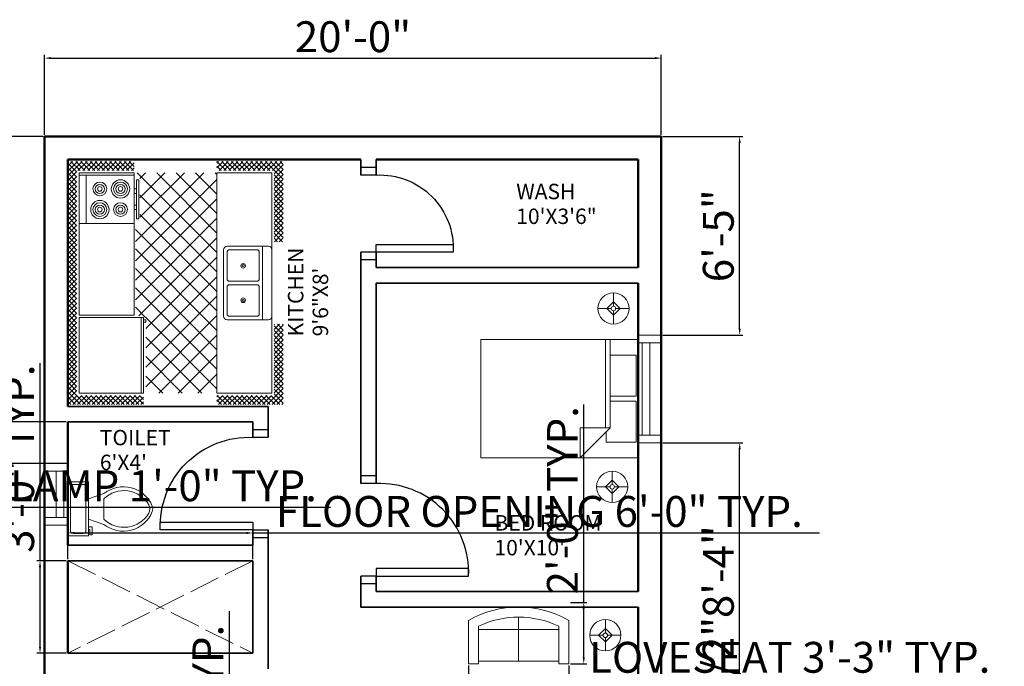
# Model space of a CAD drawing. Units: inches. Extents: x 2296 to 3335, y 495 to 1294.
# Tile 7 of 7: x 2952 to 3335, y 862 to 1113. Entities that reach past the tile are written whole.
import ezdxf

# ---------------------------------------------------------------- set-up
doc = ezdxf.new("R2010")
doc.units = ezdxf.units.IN
doc.linetypes.add('ACAD_ISO02W100', pattern=[15, 12, -3])
for name, color, linetype, lineweight in [('A-ANNO-DIMS', 2, 'Continuous', 18), ('A-AREA-IDEN', 7, 'Continuous', 18), ('A-FLOR-FIXT', 8, 'Continuous', 18), ('A-FLOR-OPEN', 7, 'ACAD_ISO02W100', 18), ('DOORS', 1, 'Continuous', 25), ('E-LITE', 2, 'Continuous', 18), ('FURNITURE', 2, 'Continuous', 18), ('INNER WALL', 6, 'Continuous', 35), ('OUTER WALL', 5, 'Continuous', 50), ('P-FIXT', 4, 'Continuous', 18), ('VENTILATOR', 4, 'Continuous', 18), ('WINDOWS', 3, 'Continuous', 18)]:
    doc.layers.add(name, color=color, linetype=linetype, lineweight=lineweight)
doc.styles.get("Standard").update_dxf_attribs({"font": 'arial.ttf'})
doc.dimstyles.new('ISO-25', dxfattribs={"dimtxt": 12, "dimasz": 2.5, "dimexe": 1.25, "dimexo": 0.625, "dimtad": 1, "dimdec": 1, "dimlunit": 3, "dimtxsty": 'Standard', "dimcen": 2.5, "dimadec": 0, "dimazin": 0, "dimtfac": 1, "dimtdec": 1, "dimtmove": 0, "dimatfit": 3, "dimfxl": 1, "dimarcsym": 0})

# ---------------------------------------------------------------- blocks, each defined once
blk = doc.blocks.new('Kitchen Layout - 7 x 8 ft')
for p, q in [((-5, 81.32), (2.68, 89)), ((-5, 83.44), (0.56, 89)), ((-5, 85.56), (-1.56, 89)), ((-5, 87.68), (-3.68, 89)), ((-1, 84.97), (-5, 88.97)), ((-1, 82.85), (-5, 86.85)), ((1.09, 85), (-2.91, 89)), ((3.21, 85), (-0.79, 89)), ((0.81, 85), (4.81, 89)), ((5.34, 85), (1.34, 89)), ((2.93, 85), (6.93, 89)), ((7.46, 85), (3.46, 89)), ((5.05, 85), (9.05, 89)), ((9.58, 85), (5.58, 89)), ((7.17, 85), (11.17, 89)), ((11.7, 85), (7.7, 89)), ((9.29, 85), (13.29, 89)), ((13.82, 85), (9.82, 89)), ((11.41, 85), (15.41, 89)), ((15.94, 85), (11.94, 89)), ((13.53, 85), (17.53, 89)), ((18.06, 85), (14.06, 89)), ((15.65, 85), (19.65, 89)), ((20.18, 85), (16.18, 89)), ((17.78, 85), (21.78, 89)), ((22.31, 85), (18.31, 89)), ((19.9, 85), (23.9, 89)), ((24.43, 85), (20.43, 89)), ((22.02, 85), (26.02, 89)), ((26.55, 85), (22.55, 89)), ((24.14, 85), (28.14, 89)), ((28.67, 85), (24.67, 89)), ((26.26, 85), (30.26, 89)), ((30.79, 85), (26.79, 89)), ((28.38, 85), (32.38, 89)), ((32.91, 85), (28.91, 89)), ((30.5, 85), (34.5, 89)), ((35.03, 85), (31.03, 89)), ((32.63, 85), (36.63, 89)), ((37.16, 85), (33.16, 89)), ((34.75, 85), (38.75, 89)), ((39.28, 85), (35.28, 89)), ((36.87, 85), (40.87, 89)), ((41.4, 85), (37.4, 89)), ((38.99, 85), (42.99, 89)), ((43.52, 85), (39.52, 89)), ((41.11, 85), (45.11, 89)), ((45.64, 85), (41.64, 89)), ((43.23, 85), (47.23, 89)), ((47.76, 85), (43.76, 89)), ((45.35, 85), (49.35, 89)), ((49.88, 85), (45.88, 89)), ((47.47, 85), (51.47, 89)), ((52, 85), (48, 89)), ((49.6, 85), (53.6, 89)), ((54.13, 85), (50.13, 89)), ((51.72, 85), (55.72, 89)), ((56.25, 85), (52.25, 89)), ((53.84, 85), (57.84, 89)), ((58.37, 85), (54.37, 89)), ((55.96, 85), (59.96, 89)), ((60.49, 85), (56.49, 89)), ((58.08, 85), (62.08, 89)), ((62.61, 85), (58.61, 89)), ((60.2, 85), (64.2, 89)), ((64.73, 85), (60.73, 89)), ((62.32, 85), (66.32, 89)), ((66.85, 85), (62.85, 89)), ((64.45, 85), (68.45, 89)), ((68.97, 85), (64.97, 89)), ((66.57, 85), (70.57, 89)), ((71.1, 85), (67.1, 89)), ((68.69, 85), (72.69, 89)), ((73.22, 85), (69.22, 89)), ((70.81, 85), (74.81, 89)), ((75.34, 85), (71.34, 89)), ((72.93, 85), (76.93, 89)), ((77.46, 85), (73.46, 89)), ((75.05, 85), (79.05, 89)), ((79.58, 85), (75.58, 89)), ((77.17, 85), (81.17, 89)), ((81.7, 85), (77.7, 89)), ((79.29, 85), (83.29, 89)), ((83.82, 85), (79.82, 89)), ((81.42, 85), (85.42, 89)), ((85.95, 85), (81.95, 89)), ((83.54, 85), (87.54, 89)), ((88.07, 85), (84.07, 89)), ((85.66, 85), (89.66, 89)), ((90.19, 85), (86.19, 89)), ((87.78, 85), (91.78, 89)), ((92.31, 85), (88.31, 89)), ((89.9, 85), (93.9, 89)), ((94.43, 85), (90.43, 89)), ((92.02, 85), (96.02, 89)), ((96.55, 85), (92.55, 89)), ((94.14, 85), (98.14, 89)), ((101, 82.67), (94.67, 89)), ((96.27, 85), (100.27, 89)), ((101, 84.79), (96.79, 89)), ((97, 83.61), (101, 87.61)), ((101, 86.92), (98.92, 89)), ((-1, 80.73), (-5, 84.73)), ((-5, 79.19), (-1, 83.19)), ((-1, 78.61), (-5, 82.61)), ((34, 84), (96, 84)), ((34, 60), (34, 84)), ((96, 84), (96, 60)), ((97, 81.49), (101, 85.49)), ((101, 80.55), (97, 84.55)), ((97, 79.37), (101, 83.37)), ((101, 78.43), (97, 82.43)), ((-5, 77.07), (-1, 81.07)), ((-1, 76.49), (-5, 80.49)), ((-5, 74.95), (-1, 78.95)), ((-1, 74.36), (-5, 78.36)), ((74, 81), (95, 81)), ((97, 77.25), (101, 81.25)), ((101, 76.31), (97, 80.31)), ((97, 75.13), (101, 79.13)), ((101, 74.19), (97, 78.19)), ((-5, 72.83), (-1, 76.83)), ((-1, 72.24), (-5, 76.24)), ((-5, 70.71), (-1, 74.71)), ((-1, 70.12), (-5, 74.12)), ((97, 73.01), (101, 77.01)), ((101, 72.07), (97, 76.07)), ((97, 70.89), (101, 74.89)), ((101, 69.95), (97, 73.95)), ((-5, 68.59), (-1, 72.59)), ((-1, 68), (-5, 72)), ((-5, 66.47), (-1, 70.47)), ((-1, 65.88), (-5, 69.88)), ((97, 68.76), (101, 72.76)), ((101, 67.82), (97, 71.82)), ((97, 66.64), (101, 70.64)), ((101, 65.7), (97, 69.7)), ((-5, 64.35), (-1, 68.35)), ((-1, 63.76), (-5, 67.76)), ((-5, 62.22), (-1, 66.22)), ((-1, 61.64), (-5, 65.64)), ((97, 64.52), (101, 68.52)), ((101, 63.58), (97, 67.58)), ((97, 62.4), (101, 66.4)), ((101, 61.46), (97, 65.46)), ((-5, 60.1), (-1, 64.1)), ((-1, 59.52), (-5, 63.52)), ((-5, 57.98), (-1, 61.98)), ((-1, 57.39), (-5, 61.39)), ((97, 60.28), (101, 64.28)), ((100.34, 60), (97, 63.34)), ((98.22, 60), (97, 61.22)), ((98.84, 60), (101, 62.16)), ((-1.73, 56), (-5, 59.27)), ((-3.85, 56), (-5, 57.15)), ((-4.86, 56), (-1, 59.86)), ((-2.74, 56), (-1, 57.74)), ((0, 57), (33, 57)), ((10.4, 24), (45.9, 59.5)), ((18.88, 24), (54.38, 59.5)), ((27.37, 24), (62.87, 59.5)), ((31, 55), (31, 56)), ((32, 56), (32, 55)), ((33.03, 55.11), (37.41, 59.5)), ((67.71, 24), (33.68, 58.04)), ((96, 60), (34, 60)), ((35.85, 24), (71.35, 59.5)), ((76.2, 24), (40.7, 59.5)), ((44.34, 24), (77.84, 57.5)), ((84.68, 24), (49.18, 59.5)), ((52.82, 24), (86.32, 57.5)), ((93.17, 24), (57.67, 59.5)), ((61.31, 24), (96, 58.69)), ((96, 29.65), (66.15, 59.5)), ((96, 38.14), (76.64, 57.5)), ((80, 60), (80, 59)), ((82, 59), (82, 60)), ((96, 46.63), (85.13, 57.5)), ((87, 59), (87, 60)), ((89, 60), (89, 59)), ((96, 55.11), (93.57, 57.54)), ((100.96, 60), (101, 60.04)), ((0, 30.57), (24.43, 55)), ((0, 39.06), (15.94, 55)), ((0, 47.54), (7.46, 55)), ((1.91, 24), (32.91, 55)), ((33.77, 24), (2.77, 55)), ((42.26, 24), (11.26, 55)), ((50.74, 24), (19.74, 55)), ((59.23, 24), (28.23, 55)), ((32, 55), (31, 55)), ((25.29, 24), (0, 49.29)), ((69.79, 24), (96, 50.21)), ((16.8, 24), (0, 40.8)), ((78.28, 24), (96, 41.72)), ((8.32, 24), (0, 32.32)), ((86.76, 24), (96, 33.24)), ((-5, 21.92), (-2.92, 24)), ((-5, 19.8), (-1, 23.8)), ((-1, 19.21), (-5, 23.21)), ((-5, 17.68), (-1, 21.68)), ((-1, 21.33), (-3.67, 24)), ((-1, 23.45), (-1.55, 24)), ((0, 24), (96, 24)), ((0, 0), (0, 24)), ((95.25, 24), (96, 24.75)), ((96, 24), (96, 0)), ((97, 22.1), (98.9, 24)), ((97, 19.97), (101, 23.97)), ((101, 19.03), (97, 23.03)), ((97, 17.85), (101, 21.85)), ((101, 21.16), (98.16, 24)), ((101, 23.28), (100.28, 24)), ((-1, 17.09), (-5, 21.09)), ((-5, 15.55), (-1, 19.55)), ((-1, 14.97), (-5, 18.97)), ((-5, 13.43), (-1, 17.43)), ((47.25, 6.5), (47.25, 18.5)), ((48.75, 18.5), (48.75, 6.5)), ((101, 16.91), (97, 20.91)), ((97, 15.73), (101, 19.73)), ((101, 14.79), (97, 18.79)), ((97, 13.61), (101, 17.61)), ((-1, 12.85), (-5, 16.85)), ((-5, 11.31), (-1, 15.31)), ((-1, 10.73), (-5, 14.73)), ((-5, 9.19), (-1, 13.19)), ((101, 12.67), (97, 16.67)), ((97, 11.49), (101, 15.49)), ((101, 10.55), (97, 14.55)), ((97, 9.37), (101, 13.37)), ((-1, 8.6), (-5, 12.6)), ((-5, 7.07), (-1, 11.07)), ((-1, 6.48), (-5, 10.48)), ((-5, 4.95), (-1, 8.95)), ((101, 8.43), (97, 12.43)), ((97, 7.25), (101, 11.25)), ((101, 6.31), (97, 10.31)), ((97, 5.12), (101, 9.12)), ((-1, 4.36), (-5, 8.36)), ((-5, 2.83), (-1, 6.83)), ((-1, 2.24), (-5, 6.24)), ((-5, 0.71), (-1, 4.71)), ((101, 4.18), (97, 8.18)), ((97, 3), (101, 7)), ((101, 2.06), (97, 6.06)), ((97, 0.88), (101, 4.88)), ((-1, 0.12), (-5, 4.12)), ((-5, -1.42), (-1, 2.58)), ((2, -5), (-5, 2)), ((-5, -3.54), (-1, 0.46)), ((96, 0), (0, 0)), ((64, 4), (32, 4)), ((93.24, -5), (101, 2.76)), ((95.36, -5), (101, 0.64)), ((101, -0.06), (97, 3.94)), ((101, -2.18), (97, 1.82)), ((-0.12, -5), (-5, -0.12)), ((-2.25, -5), (-5, -2.25)), ((-4.34, -5), (-0.34, -1)), ((-2.22, -5), (1.78, -1)), ((-0.1, -5), (3.9, -1)), ((4.12, -5), (0.12, -1)), ((2.02, -5), (6.02, -1)), ((6.24, -5), (2.24, -1)), ((4.14, -5), (8.14, -1)), ((8.36, -5), (4.36, -1)), ((6.27, -5), (10.27, -1)), ((10.48, -5), (6.48, -1)), ((8.39, -5), (12.39, -1)), ((12.6, -5), (8.6, -1)), ((10.51, -5), (14.51, -1)), ((14.73, -5), (10.73, -1)), ((12.63, -5), (16.63, -1)), ((16.85, -5), (12.85, -1)), ((14.75, -5), (18.75, -1)), ((18.97, -5), (14.97, -1)), ((16.87, -5), (20.87, -1)), ((21.09, -5), (17.09, -1)), ((18.99, -5), (22.99, -1)), ((23.21, -5), (19.21, -1)), ((21.11, -5), (25.11, -1)), ((25.33, -5), (21.33, -1)), ((23.24, -5), (27.24, -1)), ((27.45, -5), (23.45, -1)), ((25.36, -5), (29.36, -1)), ((29.57, -5), (25.57, -1)), ((27.48, -5), (30, -2.48)), ((30, -3.3), (27.7, -1)), ((30, -1.18), (29.82, -1)), ((66, -2.54), (67.54, -1)), ((66, -4.66), (69.66, -1)), ((69.88, -5), (66, -1.12)), ((67.76, -5), (66, -3.24)), ((67.78, -5), (71.78, -1)), ((72, -5), (68, -1)), ((69.9, -5), (73.9, -1)), ((74.12, -5), (70.12, -1)), ((72.03, -5), (76.03, -1)), ((76.24, -5), (72.24, -1)), ((74.15, -5), (78.15, -1)), ((78.36, -5), (74.36, -1)), ((76.27, -5), (80.27, -1)), ((80.49, -5), (76.49, -1)), ((78.39, -5), (82.39, -1)), ((82.61, -5), (78.61, -1)), ((80.51, -5), (84.51, -1)), ((84.73, -5), (80.73, -1)), ((82.63, -5), (86.63, -1)), ((86.85, -5), (82.85, -1)), ((84.75, -5), (88.75, -1)), ((88.97, -5), (84.97, -1)), ((86.88, -5), (90.88, -1)), ((91.09, -5), (87.09, -1)), ((89, -5), (93, -1)), ((93.21, -5), (89.21, -1)), ((91.12, -5), (95.12, -1)), ((95.34, -5), (91.34, -1)), ((97.46, -5), (93.46, -1)), ((99.58, -5), (95.58, -1)), ((101, -4.3), (97, -0.3)), ((97.48, -5), (101, -1.48)), ((99.6, -5), (101, -3.6)), ((-4.37, -5), (-5, -4.37)), ((29.6, -5), (30, -4.6))]:
    blk.add_line(p, q)
for points in [[(0, 56), (0, 84), (33, 84), (33, 56)], [(74, 60), (74, 84), (95, 84), (95, 60)], [(76, 58), (76, 59), (93, 59), (93, 58)]]:
    blk.add_lwpolyline(points, close=True)
for points in [[(32, 1.5), (32, 19.5)], [(33.5, 21), (62.5, 21)], [(33.5, 6.5), (33.5, 18.5)], [(34.5, 19.5), (46.25, 19.5)], [(49.75, 19.5), (61.5, 19.5)], [(62.5, 18.5), (62.5, 6.5)], [(64, 19.5), (64, 1.5)], [(46.25, 5.5), (34.5, 5.5)], [(61.5, 5.5), (49.75, 5.5)], [(62.5, 0), (33.5, 0)]]:
    blk.add_lwpolyline(points)
for centre, radius in [((80, 75), 4), ((80, 75), 3), ((89, 75), 3), ((80, 75), 2), ((80, 75), 1), ((89, 75), 2), ((89, 75), 1), ((80, 66), 3), ((89, 66), 4), ((89, 66), 3), ((80, 66), 2), ((80, 66), 1), ((89, 66), 2), ((89, 66), 1), ((40.5, 12.5), 1), ((40.5, 12.5), 0.5), ((55.5, 12.5), 1), ((55.5, 12.5), 0.5)]:
    blk.add_circle(centre, radius)
for centre, radius, start, end in [((33.5, 19.5), 1.5, 90, 180), ((34.5, 18.5), 1, 90, 180), ((46.25, 18.5), 1, 0, 90), ((49.75, 18.5), 1, 90, 180), ((61.5, 18.5), 1, 0, 90), ((62.5, 19.5), 1.5, 0, 90), ((34.5, 6.5), 1, 180, 270), ((46.25, 6.5), 1, 270, 0), ((49.75, 6.5), 1, 180, 270), ((61.5, 6.5), 1, 270, 0), ((33.5, 1.5), 1.5, 180, 270), ((62.5, 1.5), 1.5, 270, 0)]:
    blk.add_arc(centre, radius, start, end)
blk = doc.blocks.new('Toilet - top')
for p, q in [((9.5, -6), (9.5, -2)), ((-10, -8.5), (-8, -8.5)), ((-10, -9.5), (-10, -8.5)), ((-7, -9.5), (-10, -9.5)), ((-8, -8.5), (-8, -8)), ((-7, -8), (-7, -9.5)), ((-4, -8), (-6, -14)), ((4, -8), (6, -14)), ((4, -14), (-4, -14))]:
    blk.add_line(p, q)
blk.add_lwpolyline([(10.5, -8), (10.5, 0), (-10.5, 0), (-10.5, -8)], close=True)
for points in [[(-9.5, -2), (-9.5, -6)], [(8.5, -1), (-8.5, -1)], [(-8.5, -7), (8.5, -7)]]:
    blk.add_lwpolyline(points)
for centre, radius, start, end in [((-8.62, -1.88), 0.884, 81.8699, 188.1301), ((8.62, -1.88), 0.884, 351.8699, 98.1301), ((-8.62, -6.12), 0.884, 171.8699, 278.1301), ((8.62, -6.12), 0.884, 261.8699, 8.1301), ((3.52, -21.58), 12.17, 141.4691, 247.9714), ((4.2, -21.82), 11.33, 136.3677, 238.9468), ((-3.52, -21.58), 12.17, 292.0284, 38.5307), ((-4.2, -21.82), 11.33, 301.053, 43.6321), ((0, -27.88), 4, 245.7318, 294.2682), ((0, -29), 4, 254.8605, 285.1395)]:
    blk.add_arc(centre, radius, start, end)
blk = doc.blocks.new('Bed - Queen')
for p, q in [((0, -80.00003), (0, 0)), ((0, 0), (59.99999, 0)), ((59.99999, 0), (59.99999, -80.00003)), ((7.99999, -1.2), (28.79998, -1.2)), ((7.99999, -14.4), (7.99999, -1.2)), ((28.79998, -1.2), (28.79998, -14.4)), ((31.19999, -1.2), (51.99999, -1.2)), ((31.19999, -14.4), (31.19999, -1.2)), ((51.99999, -1.2), (51.99999, -16.4)), ((0, -14.4), (44.8, -14.4)), ((59.99999, -29.6), (44.8, -14.4)), ((44.8, -14.4), (44.8, -29.6)), ((44.8, -16.8), (0, -16.8)), ((51.99999, -16.4), (46.79936, -16.4)), ((44.8, -29.6), (59.99999, -29.6)), ((59.99999, -80.00003), (0, -80.00003))]:
    blk.add_line(p, q)
blk = doc.blocks.new('Lamp - Table')
for p, q in [((0, 7), (0, 1)), ((-1, 0), (-7, 0)), ((0, 3), (-3, 0)), ((-3, 0), (0, -3)), ((3, 0), (0, 3)), ((0, -3), (3, 0)), ((1, 0), (7, 0)), ((0, -1), (0, -7))]:
    blk.add_line(p, q)
for radius in [7, 1]:
    blk.add_circle((0, 0), radius)
blk = doc.blocks.new('Sofa - Roundback Loveseat 5 ft.')
for p, q in [((-24, -33.99998), (-24, -11.46958)), ((0, -32.44198), (0, -5.99998)), ((24.00004, -33.99998), (24.00004, -11.46958)), ((-23.9998, -13.38178), (23.99986, -13.38178)), ((-24, -32.44198), (24.00004, -32.44198))]:
    blk.add_line(p, q)
for points in [[(-24, -33.99998), (-30, -33.99998), (-30, -7.99998)], [(30.00004, -7.99998), (30.00004, -33.99998), (24.00004, -33.99998)]]:
    blk.add_lwpolyline(points)
for centre, radius, start, end in [((0, -60.24998), 60.24998, 60.13715, 119.8628), ((0, -61.38438), 55.38444, 64.32083, 115.6792)]:
    blk.add_arc(centre, radius, start, end)
blk = doc.blocks.new('DOOR-SINGLE-30IN')
for p, q in [((-3, 0), (-3, -6)), ((0, 0), (0, -6)), ((30, 0), (30, -6)), ((33, 0), (33, -6))]:
    blk.add_line(p, q)
blk.add_lwpolyline([(0, 0), (3, 0), (3, 30), (0, 30)], close=True)
blk.add_arc((1.5, 1.5), 28.54, 356.9872, 93.0128)
blk = doc.blocks.new('DOOR-SINGLE-36IN')
for p, q in [((0, 39), (-6, 39)), ((0, 36), (-6, 36)), ((0, 0), (-6, 0)), ((0, -3), (-6, -3))]:
    blk.add_line(p, q)
blk.add_lwpolyline([(0, 0), (36, 0), (36, 3), (0, 3)], close=True)
blk.add_arc((1.5, 1.5), 34.53, 357.5104, 92.4896)
blk = doc.blocks.new('WIN-36IN')
for p, q in [((0, 42), (9, 42)), ((0, 39), (9, 39)), ((1.5, 3), (1.5, 39)), ((4.5, 3), (4.5, 39)), ((9, 3), (0, 3)), ((9, 0), (0, 0))]:
    blk.add_line(p, q)
blk = doc.blocks.new('VENT-18IN')
for p, q in [((0, 24), (9, 24)), ((0, 21), (9, 21)), ((4.5, 21), (4.5, 3)), ((7.5, 21), (7.5, 3)), ((9, 3), (0, 3)), ((9, 0), (0, 0))]:
    blk.add_line(p, q)
blk = doc.blocks.new('FLOOR-OPENING-72X36')
for p, q in [((0, 36), (72, 0)), ((72, 36), (0, 0))]:
    blk.add_line(p, q)
blk = doc.blocks.new('*D23')
at = {"layer": 'A-ANNO-DIMS', "color": 0, "lineweight": -2, "transparency": 16777216}
for p, q in [((2970.65, 903.64), (2970.65, 915.07)), ((2973.15, 913.82), (3040.15, 913.82)), ((3042.65, 903.64), (3042.65, 915.07)), ((3042.65, 913.82), (3263.24, 913.82))]:
    blk.add_line(p, q, dxfattribs=at)
at = {"layer": 'A-ANNO-DIMS', "color": 0, "transparency": 16777216}
for points in [[(2973.15, 914.23), (2973.15, 913.4), (2970.65, 913.82)], [(3040.15, 914.23), (3040.15, 913.4), (3042.65, 913.82)]]:
    blk.add_solid(points, dxfattribs=at)
at = {"layer": 'Defpoints', "color": 0, "transparency": 16777216}
for p in [(3042.65, 913.82), (2970.65, 903.02), (3042.65, 903.02)]:
    blk.add_point(p, dxfattribs=at)
at = {"layer": 'A-ANNO-DIMS', "color": 0, "transparency": 16777216, "insert": (3154.19, 920.65), "char_height": 12, "attachment_point": 5}
blk.add_mtext('FLOOR OPENING 6\'-0" TYP.', dxfattribs=at)
blk = doc.blocks.new('*D24')
at = {"layer": 'A-ANNO-DIMS', "color": 0, "lineweight": -2, "transparency": 16777216}
for p, q in [((2959.85, 903.02), (2959.85, 979.91)), ((2970.02, 903.02), (2958.6, 903.02)), ((2959.85, 869.52), (2959.85, 900.52)), ((2970.02, 867.02), (2958.6, 867.02))]:
    blk.add_line(p, q, dxfattribs=at)
at = {"layer": 'A-ANNO-DIMS', "color": 0, "transparency": 16777216}
for points in [[(2959.43, 900.52), (2960.26, 900.52), (2959.85, 903.02)], [(2959.43, 869.52), (2960.26, 869.52), (2959.85, 867.02)]]:
    blk.add_solid(points, dxfattribs=at)
at = {"layer": 'Defpoints', "color": 0, "transparency": 16777216}
for p in [(2959.85, 903.02), (2970.65, 903.02), (2970.65, 867.02)]:
    blk.add_point(p, dxfattribs=at)
at = {"layer": 'A-ANNO-DIMS', "color": 0, "transparency": 16777216, "insert": (2953.09, 942.71), "char_height": 12, "attachment_point": 5, "rotation": 90}
blk.add_mtext('3\'-0" TYP.', dxfattribs=at)
blk = doc.blocks.new('*D29')
at = {"layer": 'A-ANNO-DIMS', "color": 0, "lineweight": -2, "transparency": 16777216}
for p, q in [((2875.48, 925.07), (2875.48, 922.62)), ((2877.98, 923.87), (2885.16, 923.87)), ((2887.66, 925.07), (2887.66, 922.62)), ((2887.66, 923.87), (3072.94, 923.87))]:
    blk.add_line(p, q, dxfattribs=at)
at = {"layer": 'A-ANNO-DIMS', "color": 0, "transparency": 16777216}
for points in [[(2877.98, 924.29), (2877.98, 923.45), (2875.48, 923.87)], [(2885.16, 924.29), (2885.16, 923.45), (2887.66, 923.87)]]:
    blk.add_solid(points, dxfattribs=at)
at = {"layer": 'Defpoints', "color": 0, "transparency": 16777216}
for p in [(2875.48, 925.7), (2887.66, 925.7), (2887.66, 923.87)]:
    blk.add_point(p, dxfattribs=at)
at = {"layer": 'A-ANNO-DIMS', "color": 0, "transparency": 16777216, "insert": (2981.55, 930.62), "char_height": 12, "attachment_point": 5}
blk.add_mtext('TABLE LAMP 1\'-0" TYP.', dxfattribs=at)
blk = doc.blocks.new('*D41')
at = {"layer": 'A-ANNO-DIMS', "color": 0, "lineweight": -2, "transparency": 16777216}
for p, q in [((3126.63, 862.3), (3126.63, 855.82)), ((3165.62, 862.3), (3165.62, 855.82)), ((3129.13, 857.07), (3163.12, 857.07)), ((3165.62, 857.07), (3335.15, 857.07))]:
    blk.add_line(p, q, dxfattribs=at)
at = {"layer": 'A-ANNO-DIMS', "color": 0, "transparency": 16777216}
for points in [[(3129.13, 857.49), (3129.13, 856.66), (3126.63, 857.07)], [(3163.12, 857.49), (3163.12, 856.66), (3165.62, 857.07)]]:
    blk.add_solid(points, dxfattribs=at)
at = {"layer": 'Defpoints', "color": 0, "transparency": 16777216}
for p in [(3126.63, 862.92), (3165.62, 862.92), (3165.62, 857.07)]:
    blk.add_point(p, dxfattribs=at)
at = {"layer": 'A-ANNO-DIMS', "color": 0, "transparency": 16777216, "insert": (3251.64, 863.91), "char_height": 12, "attachment_point": 5}
blk.add_mtext('LOVESEAT 3\'-3" TYP.', dxfattribs=at)
blk = doc.blocks.new('*D42')
at = {"layer": 'A-ANNO-DIMS', "color": 0, "lineweight": -2, "transparency": 16777216}
for p, q in [((3171.47, 886.75), (3171.47, 963.85)), ((3166.25, 886.75), (3172.72, 886.75)), ((3171.47, 865.42), (3171.47, 884.25)), ((3166.25, 862.92), (3172.72, 862.92))]:
    blk.add_line(p, q, dxfattribs=at)
at = {"layer": 'A-ANNO-DIMS', "color": 0, "transparency": 16777216}
for points in [[(3171.05, 884.25), (3171.89, 884.25), (3171.47, 886.75)], [(3171.05, 865.42), (3171.89, 865.42), (3171.47, 862.92)]]:
    blk.add_solid(points, dxfattribs=at)
at = {"layer": 'Defpoints', "color": 0, "transparency": 16777216}
for p in [(3165.62, 886.75), (3171.47, 886.75), (3165.62, 862.92)]:
    blk.add_point(p, dxfattribs=at)
at = {"layer": 'A-ANNO-DIMS', "color": 0, "transparency": 16777216, "insert": (3164.72, 926.55), "char_height": 12, "attachment_point": 5, "rotation": 90}
blk.add_mtext('2\'-0" TYP.', dxfattribs=at)
blk = doc.blocks.new('*D49')
at = {"layer": 'A-ANNO-DIMS', "color": 0, "lineweight": -2, "transparency": 16777216}
for p, q in [((3033.55, 677.03), (3033.55, 883.38)), ((3031.26, 677.03), (3034.8, 677.03)), ((3033.55, 660.07), (3033.55, 674.53)), ((3031.26, 657.57), (3034.8, 657.57))]:
    blk.add_line(p, q, dxfattribs=at)
at = {"layer": 'A-ANNO-DIMS', "color": 0, "transparency": 16777216}
for points in [[(3033.13, 674.53), (3033.97, 674.53), (3033.55, 677.03)], [(3033.13, 660.07), (3033.97, 660.07), (3033.55, 657.57)]]:
    blk.add_solid(points, dxfattribs=at)
at = {"layer": 'Defpoints', "color": 0, "transparency": 16777216}
for p in [(3030.63, 677.03), (3033.55, 677.03), (3030.63, 657.57)]:
    blk.add_point(p, dxfattribs=at)
at = {"layer": 'A-ANNO-DIMS', "color": 0, "transparency": 16777216, "insert": (3026.72, 781.45), "char_height": 12, "attachment_point": 5, "rotation": 90}
blk.add_mtext('SIDE TABLE 1\'-7 1/2" TYP.', dxfattribs=at)
blk = doc.blocks.new('*D53')
at = {"layer": 'A-ANNO-DIMS', "color": 0, "lineweight": -2, "transparency": 16777216}
for p, q in [((2961.65, 1068.64), (2961.65, 1099.77)), ((2964.15, 1098.52), (3199.15, 1098.52)), ((3201.65, 1068.64), (3201.65, 1099.77))]:
    blk.add_line(p, q, dxfattribs=at)
at = {"layer": 'A-ANNO-DIMS', "color": 0, "transparency": 16777216}
for points in [[(2964.15, 1098.93), (2964.15, 1098.1), (2961.65, 1098.52)], [(3199.15, 1098.93), (3199.15, 1098.1), (3201.65, 1098.52)]]:
    blk.add_solid(points, dxfattribs=at)
at = {"layer": 'Defpoints', "color": 0, "transparency": 16777216}
for p in [(3201.65, 1098.52), (2961.65, 1068.02), (3201.65, 1068.02)]:
    blk.add_point(p, dxfattribs=at)
at = {"layer": 'A-ANNO-DIMS', "color": 0, "transparency": 16777216, "insert": (3081.65, 1105.27), "char_height": 12, "attachment_point": 5}
blk.add_mtext('20\'-0"', dxfattribs=at)
blk = doc.blocks.new('*D54')
at = {"layer": 'A-ANNO-DIMS', "color": 0, "lineweight": -2, "transparency": 16777216}
for p, q in [((2961.02, 1068.02), (2929.9, 1068.02)), ((2931.15, 590.52), (2931.15, 1065.52)), ((2961.02, 588.02), (2929.9, 588.02))]:
    blk.add_line(p, q, dxfattribs=at)
at = {"layer": 'A-ANNO-DIMS', "color": 0, "transparency": 16777216}
for points in [[(2930.73, 1065.52), (2931.56, 1065.52), (2931.15, 1068.02)], [(2930.73, 590.52), (2931.56, 590.52), (2931.15, 588.02)]]:
    blk.add_solid(points, dxfattribs=at)
at = {"layer": 'Defpoints', "color": 0, "transparency": 16777216}
for p in [(2931.15, 1068.02), (2961.65, 1068.02), (2961.65, 588.02)]:
    blk.add_point(p, dxfattribs=at)
at = {"layer": 'A-ANNO-DIMS', "color": 0, "transparency": 16777216, "insert": (2924.39, 828.02), "char_height": 12, "attachment_point": 5, "rotation": 90}
blk.add_mtext('40\'-0"', dxfattribs=at)
blk = doc.blocks.new('*D66')
at = {"layer": 'A-ANNO-DIMS', "color": 0, "lineweight": -2, "transparency": 16777216}
for p, q in [((2931.15, 837.02), (2931.15, 872.67)), ((2970.02, 837.02), (2929.9, 837.02)), ((2931.15, 830.52), (2931.15, 834.52)), ((2970.02, 828.02), (2929.9, 828.02))]:
    blk.add_line(p, q, dxfattribs=at)
at = {"layer": 'A-ANNO-DIMS', "color": 0, "transparency": 16777216}
for points in [[(2930.73, 834.52), (2931.56, 834.52), (2931.15, 837.02)], [(2930.73, 830.52), (2931.56, 830.52), (2931.15, 828.02)]]:
    blk.add_solid(points, dxfattribs=at)
at = {"layer": 'Defpoints', "color": 0, "transparency": 16777216}
for p in [(2931.15, 837.02), (2970.65, 837.02), (2970.65, 828.02)]:
    blk.add_point(p, dxfattribs=at)
at = {"layer": 'A-ANNO-DIMS', "color": 0, "transparency": 16777216, "insert": (2924.39, 856.09), "char_height": 12, "attachment_point": 5, "rotation": 90}
blk.add_mtext('0\'-9"', dxfattribs=at)
blk = doc.blocks.new('*D73')
at = {"layer": 'A-ANNO-DIMS', "color": 0, "lineweight": -2, "transparency": 16777216}
for p, q in [((3202.27, 1068.02), (3233.4, 1068.02)), ((3232.15, 993.32), (3232.15, 1065.52)), ((3202.27, 990.82), (3233.4, 990.82))]:
    blk.add_line(p, q, dxfattribs=at)
at = {"layer": 'A-ANNO-DIMS', "color": 0, "transparency": 16777216}
for points in [[(3231.73, 1065.52), (3232.56, 1065.52), (3232.15, 1068.02)], [(3231.73, 993.32), (3232.56, 993.32), (3232.15, 990.82)]]:
    blk.add_solid(points, dxfattribs=at)
at = {"layer": 'Defpoints', "color": 0, "transparency": 16777216}
for p in [(3201.65, 1068.02), (3232.15, 1068.02), (3201.65, 990.82)]:
    blk.add_point(p, dxfattribs=at)
at = {"layer": 'A-ANNO-DIMS', "color": 0, "transparency": 16777216, "insert": (3225.39, 1029.42), "char_height": 12, "attachment_point": 5, "rotation": 90}
blk.add_mtext('6\'-5"', dxfattribs=at)
blk = doc.blocks.new('*D74')
at = {"layer": 'A-ANNO-DIMS', "color": 0, "lineweight": -2, "transparency": 16777216}
for p, q in [((3202.27, 948.82), (3233.4, 948.82)), ((3232.15, 851.25), (3232.15, 946.32)), ((3202.27, 848.75), (3233.4, 848.75))]:
    blk.add_line(p, q, dxfattribs=at)
at = {"layer": 'A-ANNO-DIMS', "color": 0, "transparency": 16777216}
for points in [[(3231.73, 946.32), (3232.56, 946.32), (3232.15, 948.82)], [(3231.73, 851.25), (3232.56, 851.25), (3232.15, 848.75)]]:
    blk.add_solid(points, dxfattribs=at)
at = {"layer": 'Defpoints', "color": 0, "transparency": 16777216}
for p in [(3201.65, 948.82), (3232.15, 948.82), (3201.65, 848.75)]:
    blk.add_point(p, dxfattribs=at)
at = {"layer": 'A-ANNO-DIMS', "color": 0, "transparency": 16777216, "insert": (3225.39, 898.79), "char_height": 12, "attachment_point": 5, "rotation": 90}
blk.add_mtext('8\'-4"', dxfattribs=at)
blk = doc.blocks.new('*D75')
at = {"layer": 'A-ANNO-DIMS', "color": 0, "lineweight": -2, "transparency": 16777216}
for p, q in [((3232.15, 806.75), (3232.15, 879.68)), ((3202.27, 806.75), (3233.4, 806.75)), ((3232.15, 761.57), (3232.15, 804.25)), ((3202.27, 759.07), (3233.4, 759.07))]:
    blk.add_line(p, q, dxfattribs=at)
at = {"layer": 'A-ANNO-DIMS', "color": 0, "transparency": 16777216}
for points in [[(3231.73, 804.25), (3232.56, 804.25), (3232.15, 806.75)], [(3231.73, 761.57), (3232.56, 761.57), (3232.15, 759.07)]]:
    blk.add_solid(points, dxfattribs=at)
at = {"layer": 'Defpoints', "color": 0, "transparency": 16777216}
for p in [(3201.65, 806.75), (3232.15, 806.75), (3201.65, 759.07)]:
    blk.add_point(p, dxfattribs=at)
at = {"layer": 'A-ANNO-DIMS', "color": 0, "transparency": 16777216, "insert": (3225.31, 844.47), "char_height": 12, "attachment_point": 5, "rotation": 90}
blk.add_mtext('3\'-11 1/2"', dxfattribs=at)
blk = doc.blocks.new('*D76')
at = {"layer": 'A-ANNO-DIMS', "color": 0, "lineweight": -2, "transparency": 16777216}
for p, q in [((2931.15, 957.02), (2931.15, 991.54)), ((2970.02, 957.02), (2929.9, 957.02)), ((2931.15, 943.31), (2931.15, 954.52)), ((2970.02, 940.81), (2929.9, 940.81))]:
    blk.add_line(p, q, dxfattribs=at)
at = {"layer": 'A-ANNO-DIMS', "color": 0, "transparency": 16777216}
for points in [[(2930.73, 954.52), (2931.56, 954.52), (2931.15, 957.02)], [(2930.73, 943.31), (2931.56, 943.31), (2931.15, 940.81)]]:
    blk.add_solid(points, dxfattribs=at)
at = {"layer": 'Defpoints', "color": 0, "transparency": 16777216}
for p in [(2931.15, 957.02), (2970.65, 957.02), (2970.65, 940.81)]:
    blk.add_point(p, dxfattribs=at)
at = {"layer": 'A-ANNO-DIMS', "color": 0, "transparency": 16777216, "insert": (2924.5, 975.53), "char_height": 12, "attachment_point": 5, "rotation": 90}
blk.add_mtext('1\'-4"', dxfattribs=at)

msp = doc.modelspace()

# ---------------------------------------------------------------- linework, layer by layer
at = {"layer": 'INNER WALL'}
for p, q in [((3084.65, 1059.02), (3084.65, 1053.02)), ((3084.65, 1059.02), (3084.65, 1053.02)), ((3090.65, 1059.02), (3090.65, 1053.02)), ((3084.65, 1023.02), (3084.65, 963.02)), ((3084.65, 1023.02), (3084.65, 933.02)), ((3090.65, 1023.02), (3090.65, 1017.02)), ((3192.65, 1017.02), (3090.65, 1017.02)), ((3192.65, 1011.02), (3090.65, 1011.02)), ((3090.65, 1011.02), (3090.65, 933.02)), ((3048.65, 963.02), (2970.65, 963.02)), ((3048.65, 963.02), (3048.65, 951.02)), ((3042.65, 957.02), (2970.65, 957.02)), ((3042.65, 957.02), (3042.65, 951.02)), ((3042.65, 915.02), (3042.65, 909.02)), ((3048.65, 915.02), (3048.65, 861.02)), ((3042.65, 909.02), (2970.65, 909.02)), ((3042.65, 903.02), (2970.65, 903.02)), ((3042.65, 903.02), (3042.65, 867.02)), ((3084.65, 897.02), (3084.65, 885.02)), ((3090.65, 897.02), (3090.65, 891.02)), ((3192.65, 891.02), (3090.65, 891.02)), ((3192.65, 885.02), (3084.65, 885.02)), ((3042.65, 867.02), (2970.65, 867.02))]:
    msp.add_line(p, q, dxfattribs=at)
at = {"layer": 'OUTER WALL'}
for p, q in [((3084.65, 1059.02), (2970.65, 1059.02)), ((2970.65, 1059.02), (2970.65, 963.02)), ((3192.65, 1059.02), (3090.65, 1059.02)), ((3192.65, 1017.02), (3192.65, 1059.02)), ((3192.65, 891.02), (3192.65, 1011.02)), ((2970.65, 957.02), (2970.65, 909.02)), ((2970.65, 903.02), (2970.65, 867.02)), ((3192.65, 783.02), (3192.65, 885.02))]:
    msp.add_line(p, q, dxfattribs=at)
msp.add_lwpolyline([(3066.65, 588.02), (3201.65, 588.02), (3201.65, 1068.02), (2961.65, 1068.02), (2961.65, 588.02), (2970.65, 588.02)], dxfattribs=at)

# ---------------------------------------------------------------- block references
at = {"layer": 'A-FLOR-FIXT', "xscale": 0.8922679191465929, "yscale": 0.8922679191465929, "zscale": 0.8922679191465929, "rotation": 90.00000000002456}
msp.add_blockref('Kitchen Layout - 7 x 8 ft', (3050.06, 968.21), dxfattribs=at)
at = {"layer": 'A-FLOR-OPEN'}
msp.add_blockref('FLOOR-OPENING-72X36', (2970.65, 867.02), dxfattribs=at)
at = {"layer": 'DOORS', "extrusion": (0, 0, -1), "zscale": -1, "rotation": 89.99999999999982}
msp.add_blockref('DOOR-SINGLE-30IN', (-3090.65, 1023.02), dxfattribs=at)
at = {"layer": 'DOORS', "extrusion": (0, 0, -1), "zscale": -1}
msp.add_blockref('DOOR-SINGLE-36IN', (-3042.65, 915.02), dxfattribs=at)
at = {"layer": 'DOORS'}
msp.add_blockref('DOOR-SINGLE-36IN', (3090.65, 897.02), dxfattribs=at)
at = {"layer": 'E-LITE', "xscale": 0.8700180084150424, "yscale": 0.8700180084150424, "zscale": 0.8700180084150424}
for p in [(3183.02, 1001.13), (3182.56, 931.79), (3179.87, 874.03)]:
    msp.add_blockref('Lamp - Table', p, dxfattribs=at)
at = {"layer": 'FURNITURE', "xscale": 0.7674836837443932, "yscale": 0.7674836837443932, "zscale": 0.7674836837443932, "rotation": 270}
msp.add_blockref('Bed - Queen', (3192.78, 989.09), dxfattribs=at)
at = {"layer": 'FURNITURE', "xscale": 0.6498910467683475, "yscale": 0.6498910467683475, "zscale": 0.6498910467683475}
msp.add_blockref('Sofa - Roundback Loveseat 5 ft.', (3146.12, 885.02), dxfattribs=at)
at = {"layer": 'P-FIXT', "rotation": 90}
msp.add_blockref('Toilet - top', (2970.69, 923.16), dxfattribs=at)
at = {"layer": 'VENTILATOR'}
msp.add_blockref('VENT-18IN', (2961.65, 916.81), dxfattribs=at)
at = {"layer": 'WINDOWS'}
msp.add_blockref('WIN-36IN', (3192.65, 948.82), dxfattribs=at)

# ---------------------------------------------------------------- texts
at = {"layer": 'A-AREA-IDEN'}
for s, p in [('WASH', (3145.2, 1043.63)), ('10\'X3\'6"', (3145.2, 1033.99)), ('TOILET', (2983.13, 947.92)), ("6'X4'", (2983.13, 938.28)), ('BED ROOM', (3136.74, 914.76)), ("10'X10'", (3136.74, 905.12))]:
    msp.add_text(s, height=6, dxfattribs=at).set_placement(p)
for s, p in [('KITCHEN', (3062.34, 990.28)), ('9\'6"X8\'', (3071.98, 990.28))]:
    msp.add_text(s, height=6, rotation=90, dxfattribs=at).set_placement(p)

# ---------------------------------------------------------------- dimensions: what is measured, and where the dimension line sits
at = {"layer": 'A-ANNO-DIMS'}
dim = msp.add_linear_dim(base=(3201.65, 1098.52), p1=(2961.65, 1068.02), p2=(3201.65, 1068.02), dimstyle='ISO-25', override={"dimdec": 1, "dimlfac": 1, "dimrnd": 0, "dimzin": 1, "dimdsep": 46, "dimlunit": 4, "dimfrac": 2}, dxfattribs=at)
dim.commit()
dim.dimension.update_dxf_attribs({"geometry": '*D53', "text_midpoint": (3081.65, 1105.27)})
for base, p1, p2, picture, middle in [((2931.15, 1068.02), (2961.65, 588.02), (2961.65, 1068.02), '*D54', (2924.39, 828.02)), ((3232.15, 1068.02), (3201.65, 990.82), (3201.65, 1068.02), '*D73', (3225.39, 1029.42)), ((2931.15, 957.02), (2970.65, 940.81), (2970.65, 957.02), '*D76', (2924.5, 975.53)), ((3232.15, 948.82), (3201.65, 848.75), (3201.65, 948.82), '*D74', (3225.39, 898.79)), ((3232.15, 806.75), (3201.65, 759.07), (3201.65, 806.75), '*D75', (3225.31, 844.47)), ((2931.15, 837.02), (2970.65, 828.02), (2970.65, 837.02), '*D66', (2924.39, 856.09))]:
    dim = msp.add_linear_dim(base=base, p1=p1, p2=p2, angle=90, dimstyle='ISO-25', override={"dimdec": 1, "dimlfac": 1, "dimrnd": 0, "dimzin": 1, "dimdsep": 46, "dimlunit": 4, "dimfrac": 2}, dxfattribs=at)
    dim.commit()
    dim.dimension.update_dxf_attribs({"geometry": picture, "text_midpoint": middle})
for base, p1, p2, text, picture, middle in [((2959.85, 903.02), (2970.65, 867.02), (2970.65, 903.02), '<> TYP.', '*D24', (2953.09, 942.71)), ((3171.47, 886.75), (3165.62, 862.92), (3165.62, 886.75), '<> TYP.', '*D42', (3164.72, 926.55)), ((3033.55, 677.03), (3030.63, 657.57), (3030.63, 677.03), 'SIDE TABLE <> TYP.', '*D49', (3026.72, 781.45))]:
    dim = msp.add_linear_dim(base=base, p1=p1, p2=p2, angle=90, text=text, dimstyle='ISO-25', override={"dimdec": 1, "dimlfac": 1, "dimrnd": 0, "dimzin": 1, "dimdsep": 46, "dimlunit": 4, "dimfrac": 2}, dxfattribs=at)
    dim.commit()
    dim.dimension.update_dxf_attribs({"geometry": picture, "text_midpoint": middle})
for base, p1, p2, text, picture, middle in [((2887.66, 923.87), (2875.48, 925.7), (2887.66, 925.7), 'TABLE LAMP <> TYP.', '*D29', (2981.55, 930.62)), ((3042.65, 913.82), (2970.65, 903.02), (3042.65, 903.02), 'FLOOR OPENING <> TYP.', '*D23', (3154.19, 920.65)), ((3165.62, 857.07), (3126.63, 862.92), (3165.62, 862.92), 'LOVESEAT <> TYP.', '*D41', (3251.64, 863.91))]:
    dim = msp.add_linear_dim(base=base, p1=p1, p2=p2, text=text, dimstyle='ISO-25', override={"dimdec": 1, "dimlfac": 1, "dimrnd": 0, "dimzin": 1, "dimdsep": 46, "dimlunit": 4, "dimfrac": 2}, dxfattribs=at)
    dim.commit()
    dim.dimension.update_dxf_attribs({"geometry": picture, "text_midpoint": middle})

doc.saveas('drawing.dxf')
